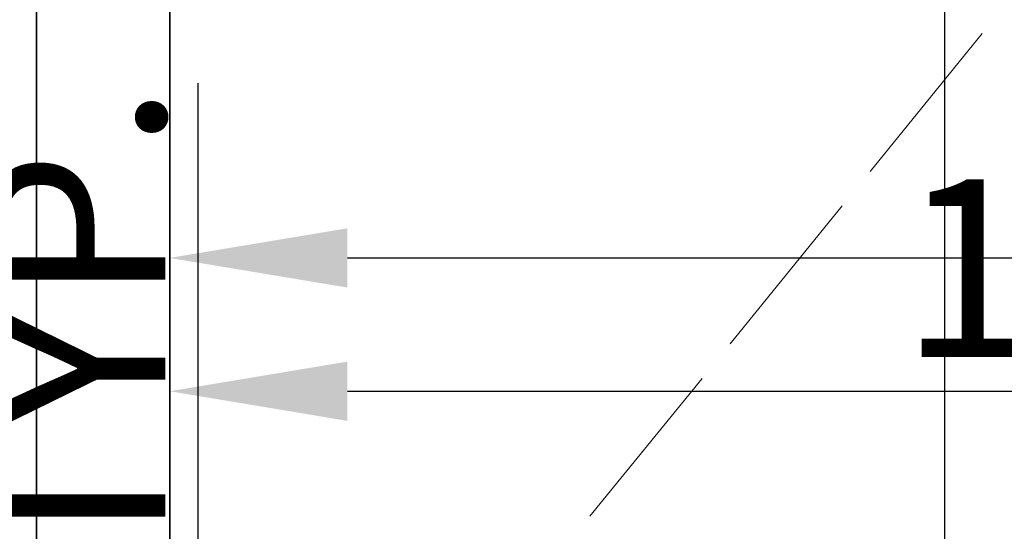
# Model space of a CAD drawing. Units: inches. Extents: x 2083 to 3317, y 1141 to 2115.
# Tile 80 of 256: x 2226 to 2292, y 1512 to 1546. Entities that reach past the tile are written whole.
import ezdxf

# ---------------------------------------------------------------- set-up
doc = ezdxf.new("R2010")
doc.units = ezdxf.units.IN
doc.linetypes.add('ACAD_ISO02W100', pattern=[15, 12, -3])
for name, color, linetype, lineweight in [('A-ANNO-DIMS', 2, 'Continuous', 18), ('A-FLOR-OPEN', 8, 'ACAD_ISO02W100', 13), ('A-WALL', 7, 'Continuous', 35)]:
    doc.layers.add(name, color=color, linetype=linetype, lineweight=lineweight)
doc.layers.add('A-WALL-PATT', color=251, linetype='Continuous', lineweight=13, true_color=0x636466)
doc.styles.get("Standard").update_dxf_attribs({"font": 'arial.ttf'})
doc.dimstyles.new('ISO-25', dxfattribs={"dimtxt": 12, "dimasz": 12, "dimexe": 1.25, "dimexo": 0.625, "dimtad": 1, "dimlunit": 3, "dimtxsty": 'Standard', "dimcen": 2.5, "dimadec": 0, "dimazin": 0, "dimtfac": 1, "dimtmove": 0, "dimatfit": 3, "dimfxl": 1, "dimarcsym": 0})

# ---------------------------------------------------------------- blocks, each defined once
blk = doc.blocks.new('*D31')
at = {"layer": 'A-ANNO-DIMS', "color": 0, "lineweight": -2, "transparency": 16777216}
for p, q in [((2237.871, 1456.649), (2237.871, 1541.915)), ((2239.393, 1444.649), (2236.621, 1444.649)), ((2237.871, 1431.548), (2237.871, 1444.649)), ((2239.393, 1431.548), (2236.621, 1431.548)), ((2237.871, 1419.548), (2237.871, 1407.548))]:
    blk.add_line(p, q, dxfattribs=at)
at = {"layer": 'A-ANNO-DIMS', "color": 0, "transparency": 16777216}
for points in [[(2235.871, 1456.649), (2239.871, 1456.649), (2237.871, 1444.649)], [(2235.871, 1419.548), (2239.871, 1419.548), (2237.871, 1431.548)]]:
    blk.add_solid(points, dxfattribs=at)
at = {"layer": 'Defpoints', "color": 0, "transparency": 16777216}
for p in [(2237.871, 1444.649), (2240.018, 1444.649), (2240.018, 1431.548)]:
    blk.add_point(p, dxfattribs=at)
at = {"layer": 'A-ANNO-DIMS', "color": 0, "transparency": 16777216, "insert": (2231.217, 1505.282), "char_height": 12, "attachment_point": 5, "rotation": 90}
blk.add_mtext('1\'-1" TYP.', dxfattribs=at)
blk = doc.blocks.new('*D45')
at = {"layer": 'A-ANNO-DIMS', "color": 0, "lineweight": -2, "transparency": 16777216}
for p, q in [((2235.96, 1478.386), (2235.96, 1531.361)), ((2418.96, 1478.386), (2418.96, 1531.361)), ((2247.96, 1530.111), (2406.96, 1530.111))]:
    blk.add_line(p, q, dxfattribs=at)
at = {"layer": 'A-ANNO-DIMS', "color": 0, "transparency": 16777216}
for points in [[(2247.96, 1532.111), (2247.96, 1528.111), (2235.96, 1530.111)], [(2406.96, 1532.111), (2406.96, 1528.111), (2418.96, 1530.111)]]:
    blk.add_solid(points, dxfattribs=at)
at = {"layer": 'Defpoints', "color": 0, "transparency": 16777216}
for p in [(2418.96, 1530.111), (2235.96, 1477.761), (2418.96, 1477.761)]:
    blk.add_point(p, dxfattribs=at)
at = {"layer": 'A-ANNO-DIMS', "color": 0, "transparency": 16777216, "insert": (2327.46, 1536.867), "char_height": 12, "attachment_point": 5}
blk.add_mtext('15\'-3"', dxfattribs=at)
blk = doc.blocks.new('*D62')
at = {"layer": 'A-ANNO-DIMS', "color": 0, "lineweight": -2, "transparency": 16777216}
for p, q in [((2235.96, 1469.386), (2235.96, 1522.361)), ((2379.96, 1469.386), (2379.96, 1522.361)), ((2247.96, 1521.111), (2367.96, 1521.111))]:
    blk.add_line(p, q, dxfattribs=at)
at = {"layer": 'A-ANNO-DIMS', "color": 0, "transparency": 16777216}
for points in [[(2247.96, 1523.111), (2247.96, 1519.111), (2235.96, 1521.111)], [(2367.96, 1523.111), (2367.96, 1519.111), (2379.96, 1521.111)]]:
    blk.add_solid(points, dxfattribs=at)
at = {"layer": 'Defpoints', "color": 0, "transparency": 16777216}
for p in [(2379.96, 1521.111), (2235.96, 1468.761), (2379.96, 1468.761)]:
    blk.add_point(p, dxfattribs=at)
at = {"layer": 'A-ANNO-DIMS', "color": 0, "transparency": 16777216, "insert": (2307.96, 1527.863), "char_height": 12, "attachment_point": 5}
blk.add_mtext('12\'-0"', dxfattribs=at)
blk = doc.blocks.new('*D64')
at = {"layer": 'A-ANNO-DIMS', "color": 0, "lineweight": -2, "transparency": 16777216}
for p, q in [((2236.585, 1702.761), (2289.56, 1702.761)), ((2288.31, 1690.761), (2288.31, 1489.761)), ((2236.585, 1477.761), (2289.56, 1477.761))]:
    blk.add_line(p, q, dxfattribs=at)
at = {"layer": 'A-ANNO-DIMS', "color": 0, "transparency": 16777216}
for points in [[(2286.31, 1690.761), (2290.31, 1690.761), (2288.31, 1702.761)], [(2286.31, 1489.761), (2290.31, 1489.761), (2288.31, 1477.761)]]:
    blk.add_solid(points, dxfattribs=at)
at = {"layer": 'Defpoints', "color": 0, "transparency": 16777216}
for p in [(2235.96, 1702.761), (2235.96, 1477.761), (2288.31, 1477.761)]:
    blk.add_point(p, dxfattribs=at)
at = {"layer": 'A-ANNO-DIMS', "color": 0, "transparency": 16777216, "insert": (2281.558, 1590.261), "char_height": 12, "attachment_point": 5, "rotation": 90}
blk.add_mtext('18\'-9"', dxfattribs=at)

msp = doc.modelspace()

# ---------------------------------------------------------------- hatches: boundary and pattern name
at = {"layer": 'A-WALL-PATT'}
h = msp.add_hatch(color=256, dxfattribs=at)
h.dxf.hatch_style = 1
h.paths.add_polyline_path([(3126.96, 2020.761), (2748.96, 2020.761), (2604.96, 2020.761), (2226.96, 2020.761), (2226.96, 1702.761), (2466.96, 1702.761), (2466.96, 1582.761), (2418.96, 1582.761), (2418.96, 1477.761), (2226.96, 1477.761), (2226.96, 1263.261), (2544.96, 1263.261), (2544.96, 1411.761), (2604.96, 1411.761), (2685.96, 1411.761), (2685.96, 1420.761), (2604.96, 1420.761), (2604.96, 1573.761), (2604.96, 1702.761), (2604.96, 2011.761), (2748.96, 2011.761), (2748.96, 1702.761), (2862.96, 1702.761), (2862.96, 1621.761), (2871.96, 1621.761), (2871.96, 1702.761), (2883.96, 1702.761), (2883.96, 1706.939, -0.026459), (2883.96, 1711.761), (2757.96, 1711.761), (2757.96, 1807.761), (2787.96, 1807.761), (2787.96, 1812.261), (2757.96, 1812.261), (2757.96, 2011.761), (2877.96, 2011.761), (2877.96, 1812.261), (2847.96, 1812.261), (2847.96, 1807.761), (2889.836, 1807.761), (2889.836, 1812.261), (2882.46, 1812.261), (2882.46, 2011.761), (3117.96, 2011.761), (3117.96, 1812.261), (2937.836, 1812.261), (2937.836, 1807.761), (2995.71, 1807.761), (2995.71, 1796.118), (3000.21, 1796.118), (3000.21, 1807.761), (3117.96, 1807.761), (3117.96, 1711.761), (3000.21, 1711.761), (3000.21, 1760.118), (2998.573, 1760.118, -0.020711), (2995.71, 1760.118), (2995.71, 1711.761), (2931.96, 1711.761), (2931.96, 1702.761), (3126.96, 1702.761)])
h.paths.add_polyline_path([(2471.46, 2011.761), (2471.46, 1810.011), (2462.717, 1810.011), (2462.717, 1805.511), (2505.96, 1805.511), (2505.96, 1810.011), (2475.96, 1810.011), (2475.96, 2011.761), (2595.96, 2011.761), (2595.96, 1810.011), (2565.96, 1810.011), (2565.96, 1805.511), (2595.96, 1805.511), (2595.96, 1711.761), (2235.96, 1711.761), (2235.96, 1805.511), (2353.71, 1805.511), (2353.71, 1796.054), (2358.21, 1796.054), (2358.21, 1805.511), (2414.717, 1805.511), (2414.717, 1810.011), (2235.96, 1810.011), (2235.96, 2011.761)], flags=16)
h.paths.add_polyline_path([(2270.205, 1994.61), (2270.205, 1970.61), (2246.205, 1970.61), (2246.205, 1994.61)], flags=0)
edge = h.paths.add_edge_path(flags=0)
edge.add_ellipse((2332.027, 1899.798), major_axis=(-3.043, 3.043), ratio=0.168252, start_angle=-161.33217, end_angle=-156.30711, ccw=False)
edge.add_ellipse((2333.082, 1898.744), major_axis=(-1.055, 1.055), ratio=0.453532, start_angle=-123.37102, end_angle=-94.15911)
edge = h.paths.add_edge_path(flags=0)
edge.add_ellipse((2332.027, 1968.876), major_axis=(3.043, 3.043), ratio=0.168252, start_angle=18.66783, end_angle=23.69289)
edge.add_spline(control_points=[(2332.926, 1970.691), (2332.227, 1970.336), (2330.894, 1969.659), (2328.413, 1970.932), (2327.204, 1967.749), (2324.71, 1969.956), (2322.533, 1967.012), (2320.013, 1971.296), (2317.68, 1968.158), (2316.041, 1967.102), (2315.427, 1966.81)], knot_values=[0, 0, 0, 0, 2.267059, 4.324559, 6.685584, 8.878641, 11.121502, 14.300359, 17.755284, 19.732645, 19.732645, 19.732645, 19.732645], degree=3, periodic=0)
edge.add_ellipse((2332.027, 1968.876), major_axis=(3.043, 3.043), ratio=0.168252, start_angle=18.66783, end_angle=23.69289, ccw=False)
edge.add_ellipse((2333.082, 1969.931), major_axis=(1.055, 1.055), ratio=0.453532, start_angle=56.62898, end_angle=85.84089, ccw=False)
edge = h.paths.add_edge_path(flags=0)
edge.add_spline(control_points=[(2296.428, 1967.988), (2293.628, 1965.336), (2287.704, 1959.727), (2299.744, 1949.996), (2294.533, 1935.669), (2290.573, 1920.604), (2293.394, 1909.974), (2296.185, 1904.967)], knot_values=[0.099185, 0.099185, 0.099185, 0.099185, 0.345301, 0.619822, 0.982653, 1.386093, 1.810555, 1.810555, 1.810555, 1.810555], degree=3, periodic=0)
edge.add_spline(control_points=[(2296.185, 1904.967), (2297.384, 1902.619), (2298.001, 1901.949), (2298.553, 1901.468)], knot_values=[0.006246, 0.006246, 0.006246, 0.006246, 0.055476, 0.055476, 0.055476, 0.055476], degree=3, periodic=0)
edge.add_spline(control_points=[(2298.553, 1901.468), (2297.259, 1900.923), (2295.225, 1900.232), (2293.06, 1900.614), (2292.101, 1900.788), (2292.09, 1900.791)], knot_values=[0.312835, 0.312835, 0.312835, 0.312835, 0.40178, 0.474987, 0.475903, 0.475903, 0.475903, 0.475903], degree=3, periodic=0)
edge.add_arc((2292.794, 1904.664), 3.937, 215.4209, 259.69818, ccw=False)
edge.add_spline(control_points=[(2289.585, 1902.382), (2289.477, 1902.535), (2289.368, 1902.688), (2289.261, 1902.841)], knot_values=[0.102872, 0.102872, 0.102872, 0.102872, 0.116896, 0.116896, 0.116896, 0.116896], degree=3, periodic=0)
edge.add_spline(control_points=[(2289.261, 1902.841), (2288.687, 1902.55), (2287.64, 1902.02), (2285.881, 1901.874), (2283.853, 1901.504), (2281.72, 1899.711), (2278.467, 1899.493), (2276.157, 1901.883), (2272.259, 1899.804), (2267.778, 1901.843), (2262.244, 1900.184), (2257.415, 1901.782), (2254.318, 1900.726), (2253.178, 1900.337)], knot_values=[0, 0, 0, 0, 1.907977, 3.477176, 5.261074, 7.972851, 11.680248, 13.717921, 16.939592, 22.789562, 27.502503, 33.595215, 37.145618, 37.145618, 37.145618, 37.145618], degree=3, periodic=0)
edge.add_line((2253.178, 1900.337), (2250.244, 1902.841))
edge.add_line((2250.244, 1902.841), (2250.244, 1965.833))
edge.add_line((2250.244, 1965.833), (2253.178, 1968.337))
edge.add_spline(control_points=[(2253.178, 1968.337), (2254.318, 1967.948), (2257.415, 1966.892), (2262.244, 1968.49), (2267.778, 1966.831), (2271.527, 1968.537), (2273.876, 1967.828), (2274.207, 1967.728)], knot_values=[0, 0, 0, 0, 0.09018, 0.244935, 0.364644, 0.513233, 0.537855, 0.537855, 0.537855, 0.537855], degree=3, periodic=0)
edge.add_arc((2274.353, 1963.793), 3.937, 72.05113, 92.12795, ccw=False)
edge.add_arc((2281.297, 1985.23), 18.596, 252.05113, 288.56572)
edge.add_arc((2292.317, 1956.029), 12.646, 71.02679, 113.77822, ccw=False)
edge = h.paths.add_edge_path(flags=0)
edge.add_spline(control_points=[(2274.899, 1951.856), (2275.066, 1951.617), (2275.233, 1951.377), (2275.398, 1951.136)], knot_values=[1.409916, 1.409916, 1.409916, 1.409916, 1.43159, 1.43159, 1.43159, 1.43159], degree=3, periodic=0)
edge.add_spline(control_points=[(2275.398, 1951.136), (2275.792, 1950.562), (2276.179, 1949.984), (2276.546, 1949.397)], knot_values=[1.358238, 1.358238, 1.358238, 1.358238, 1.409916, 1.409916, 1.409916, 1.409916], degree=3, periodic=0)
edge.add_line((2276.546, 1949.397), (2277.437, 1947.862))
edge.add_spline(control_points=[(2277.437, 1947.862), (2276.304, 1945.673), (2274.64, 1942.427), (2274.632, 1938.094), (2272.799, 1930.852), (2274.356, 1943.897), (2275.948, 1947.923), (2276.546, 1949.397)], knot_values=[0.005632, 0.005632, 0.005632, 0.005632, 0.186014, 0.266002, 0.357087, 0.59639, 0.739732, 0.739732, 0.739732, 0.739732], degree=3, periodic=0)
edge.add_spline(control_points=[(2276.546, 1949.397), (2276.179, 1949.984), (2275.792, 1950.562), (2275.398, 1951.136)], knot_values=[1.358238, 1.358238, 1.358238, 1.358238, 1.409916, 1.409916, 1.409916, 1.409916], degree=3, periodic=0)
edge.add_spline(control_points=[(2275.398, 1951.136), (2274.943, 1950.08), (2274.208, 1948.025), (2273.935, 1944.851), (2272.469, 1937.627), (2273.466, 1945.696), (2274.701, 1951.059), (2274.899, 1951.856)], knot_values=[0.104364, 0.104364, 0.104364, 0.104364, 0.189636, 0.269624, 0.36071, 0.600013, 0.644622, 0.644622, 0.644622, 0.644622], degree=3, periodic=0)
h.paths.add_polyline_path([(2269.168, 1963.128, -0.357527), (2268.171, 1960.976, -0.092561), (2268.171, 1939.436, -0.357527), (2269.168, 1937.285, -0.357527), (2267.016, 1938.282, -0.164785), (2254.686, 1938.282, -0.357527), (2252.534, 1937.285, -0.357527), (2253.531, 1939.436, -0.092561), (2253.531, 1960.976, -0.357527), (2252.534, 1963.128, -0.357527), (2254.686, 1962.131, -0.164785), (2267.016, 1962.131, -0.357527)], flags=0)
h.paths.add_polyline_path([(2248.874, 1967.802), (2248.874, 1957.028), (2249.458, 1957.028), (2249.458, 1911.647), (2248.874, 1911.647), (2248.874, 1900.873), (2246.512, 1900.873, 0.197327), (2244.15, 1902.457), (2244.15, 1966.218, 0.197327), (2246.512, 1967.802)], flags=0)
h.paths.add_polyline_path([(2269.168, 1931.389, -0.357527), (2268.171, 1929.238, -0.092561), (2268.171, 1907.698, -0.357527), (2269.168, 1905.547, -0.357527), (2267.016, 1906.544, -0.164785), (2254.686, 1906.544, -0.357527), (2252.534, 1905.547, -0.357527), (2253.531, 1907.698, -0.092561), (2253.531, 1929.238, -0.357527), (2252.534, 1931.389, -0.357527), (2254.686, 1930.392, -0.164785), (2267.016, 1930.392, -0.357527)], flags=0)
edge = h.paths.add_edge_path(flags=0)
edge.add_spline(control_points=[(2276.197, 1906.724), (2276.168, 1909.029), (2276.114, 1913.372), (2270.598, 1924.925), (2273.905, 1919.013), (2275.922, 1916.262), (2275.475, 1912.402), (2277.258, 1910.381), (2276.696, 1908.225), (2276.646, 1906.813), (2276.618, 1906.008)], knot_values=[0, 0, 0, 0, 8.61026, 16.221274, 18.843057, 23.804898, 27.440828, 29.356102, 31.203478, 33.650687, 33.650687, 33.650687, 33.650687], degree=3, periodic=0)
edge.add_spline(control_points=[(2276.618, 1906.008), (2276.623, 1905.624), (2276.498, 1904.629), (2275.442, 1903.855), (2274.937, 1903.08), (2274.859, 1902.841)], knot_values=[0.156488, 0.156488, 0.156488, 0.156488, 0.184398, 0.231376, 0.250598, 0.250598, 0.250598, 0.250598], degree=3, periodic=0)
edge.add_line((2274.859, 1902.841), (2276.506, 1902.841))
edge.add_spline(control_points=[(2276.506, 1902.841), (2276.788, 1903.085), (2277.665, 1904.125), (2278.25, 1904.341), (2277.654, 1908.527), (2278.156, 1906.228), (2278.1, 1905.286), (2278.847, 1904.069), (2277.857, 1903.415), (2277.874, 1902.991), (2277.904, 1902.841)], knot_values=[0.059574, 0.059574, 0.059574, 0.059574, 0.080753, 0.103741, 0.16972, 0.176036, 0.207137, 0.240474, 0.262341, 0.27366, 0.27366, 0.27366, 0.27366], degree=3, periodic=0)
edge.add_line((2277.904, 1902.841), (2280.03, 1902.841))
edge.add_spline(control_points=[(2280.03, 1902.841), (2279.888, 1903.088), (2279.499, 1903.982), (2280.152, 1905.939), (2278.104, 1909.658), (2279.762, 1907.185), (2280.328, 1904.875), (2280.485, 1903.49), (2281.463, 1903.249), (2281.758, 1902.936), (2281.834, 1902.841)], knot_values=[0.013856, 0.013856, 0.013856, 0.013856, 0.034874, 0.088867, 0.107879, 0.126738, 0.158714, 0.193757, 0.217487, 0.226722, 0.226722, 0.226722, 0.226722], degree=3, periodic=0)
edge.add_spline(control_points=[(2281.834, 1902.841), (2281.788, 1902.827), (2281.647, 1902.783), (2281.396, 1902.859), (2281.088, 1902.985), (2280.721, 1903.061), (2280.333, 1903.026), (2280.125, 1902.899), (2280.03, 1902.841)], knot_values=[0, 0, 0, 0, 0.14413, 0.435517, 0.749276, 1.153046, 1.548371, 1.878348, 1.878348, 1.878348, 1.878348], degree=3, periodic=0)
edge.add_line((2280.03, 1902.841), (2277.904, 1902.841))
edge.add_spline(control_points=[(2277.904, 1902.841), (2277.893, 1902.796), (2277.865, 1902.68), (2277.607, 1902.687), (2277.274, 1902.801), (2276.838, 1902.62), (2276.584, 1902.789), (2276.506, 1902.841)], knot_values=[0, 0, 0, 0, 0.127189, 0.326199, 0.628009, 1.24357, 1.515331, 1.515331, 1.515331, 1.515331], degree=3, periodic=0)
edge.add_line((2276.506, 1902.841), (2274.859, 1902.841))
edge.add_spline(control_points=[(2274.859, 1902.841), (2274.814, 1902.899), (2274.725, 1903.013), (2274.493, 1903.119), (2274.244, 1902.961), (2273.937, 1903.185), (2273.614, 1902.983), (2273.408, 1902.883), (2273.322, 1902.841)], knot_values=[0, 0, 0, 0, 0.21843, 0.436957, 0.687977, 0.990379, 1.398396, 1.69185, 1.69185, 1.69185, 1.69185], degree=3, periodic=0)
edge.add_spline(control_points=[(2273.322, 1902.841), (2273.617, 1903.446), (2274.274, 1904.538), (2276.027, 1904.574), (2276.207, 1906.584), (2276.197, 1906.724)], knot_values=[0.012227, 0.012227, 0.012227, 0.012227, 0.059472, 0.106218, 0.134458, 0.134458, 0.134458, 0.134458], degree=3, periodic=0)
h.paths.add_polyline_path([(2270.776, 1897.79), (2270.776, 1873.79), (2246.776, 1873.79), (2246.776, 1897.79)], flags=0)
h.paths.add_polyline_path([(2353.71, 1760.005), (2353.71, 1760.054), (2358.21, 1760.054, -0.033729)], flags=0)
h.paths.add_polyline_path([(2321.819, 1737.529), (2341.995, 1737.529, -0.414214), (2343.203, 1736.321), (2343.203, 1721.021, -0.414214), (2341.995, 1719.813), (2321.819, 1719.813, -0.414214), (2320.611, 1721.021), (2320.611, 1736.321, -0.414214)], flags=0)
h.paths.add_polyline_path([(2324.235, 1736.321), (2339.579, 1736.321, -0.414214), (2341.995, 1733.905), (2341.995, 1725.45, -0.414214), (2339.579, 1723.034), (2333.681, 1723.034), (2333.845, 1722.045, -0.870646), (2335.425, 1721.826, -0.767327), (2333.923, 1721.423), (2331.291, 1721.423, -0.767327), (2329.788, 1721.826, -0.870646), (2331.368, 1722.045), (2331.533, 1723.034), (2324.235, 1723.034, -0.414214), (2321.819, 1725.45), (2321.819, 1733.905, -0.414214)], flags=0)
h.paths.add_polyline_path([(2570.484, 1928.615), (2589.684, 1928.615), (2590.169, 1928.615), (2590.169, 1904.993), (2570.484, 1904.993)], flags=0)
h.paths.add_polyline_path([(2574.447, 1927.264, -1), (2572.829, 1927.264, -1)], flags=0)
h.paths.add_polyline_path([(2573.09, 1926.941), (2573.925, 1927.776), (2574.148, 1927.553), (2573.313, 1926.718)], flags=0)
h.paths.add_polyline_path([(2578.779, 1919.73, -1), (2571.592, 1919.73, -1)], flags=0)
h.paths.add_polyline_path([(2578.385, 1919.73, -1), (2571.985, 1919.73, -1)], flags=0)
h.paths.add_polyline_path([(2331.596, 1729.476, -1), (2333.618, 1729.476, -1)], flags=0)
h.paths.add_polyline_path([(2578.034, 1927.264, -1), (2576.416, 1927.264, -1)], flags=0)
h.paths.add_polyline_path([(2576.689, 1927.531), (2576.912, 1927.754), (2577.747, 1926.919), (2577.524, 1926.696)], flags=0)
h.paths.add_polyline_path([(2578.139, 1909.86, -1), (2572.232, 1909.86, -1)], flags=0)
h.paths.add_polyline_path([(2577.745, 1909.86, -1), (2572.625, 1909.86, -1)], flags=0)
h.paths.add_polyline_path([(2583.798, 1927.264, -1), (2582.179, 1927.264, -1)], flags=0)
h.paths.add_polyline_path([(2582.719, 1927.754), (2583.554, 1926.919), (2583.331, 1926.696), (2582.496, 1927.531)], flags=0)
h.paths.add_polyline_path([(2582.496, 1927.531), (2582.719, 1927.754), (2583.554, 1926.919), (2583.331, 1926.696)], flags=0)
h.paths.add_polyline_path([(2587.739, 1920.53, -1), (2581.832, 1920.53, -1)], flags=0)
h.paths.add_polyline_path([(2587.345, 1920.53, -1), (2582.225, 1920.53, -1)], flags=0)
h.paths.add_polyline_path([(2587.385, 1927.264, -1), (2585.766, 1927.264, -1)], flags=0)
h.paths.add_polyline_path([(2586.082, 1926.98), (2586.917, 1927.815), (2587.14, 1927.593), (2586.305, 1926.758)], flags=0)
h.paths.add_polyline_path([(2588.379, 1910.66, -1), (2581.192, 1910.66, -1)], flags=0)
h.paths.add_polyline_path([(2587.985, 1910.66, -1), (2581.585, 1910.66, -1)], flags=0)
h.paths.add_polyline_path([(2417.168, 1729.478), (2437.344, 1729.478, -0.414214), (2438.552, 1728.27), (2438.552, 1712.969, -0.414214), (2437.344, 1711.761), (2417.168, 1711.761, -0.414214), (2415.96, 1712.969), (2415.96, 1728.27, -0.414214)], flags=0)
h.paths.add_polyline_path([(2419.584, 1728.27), (2434.928, 1728.27, -0.414214), (2437.344, 1725.854), (2437.344, 1717.398, -0.414214), (2434.928, 1714.983), (2429.029, 1714.983), (2429.194, 1713.994, -0.870646), (2430.774, 1713.775, -0.767327), (2429.271, 1713.372), (2426.64, 1713.372, -0.767327), (2425.137, 1713.775, -0.870646), (2426.717, 1713.994), (2426.882, 1714.983), (2419.584, 1714.983, -0.414214), (2417.168, 1717.398), (2417.168, 1725.854, -0.414214)], flags=0)
h.paths.add_polyline_path([(2419.584, 1728.27), (2434.928, 1728.27, -0.414214), (2437.344, 1725.854), (2437.344, 1717.398, -0.414214), (2434.928, 1714.983), (2429.029, 1714.983), (2428.358, 1719.009), (2427.553, 1719.009), (2426.882, 1714.983), (2419.584, 1714.983, -0.414214), (2417.168, 1717.398), (2417.168, 1725.854, -0.414214)], flags=0)
h.paths.add_polyline_path([(2426.944, 1721.425, -1), (2428.967, 1721.425, -1)], flags=0)
h.paths.add_polyline_path([(2475.96, 1702.761), (2595.96, 1702.761), (2595.96, 1582.761), (2475.96, 1582.761)], flags=16)
h.paths.add_polyline_path([(2427.96, 1573.761), (2595.96, 1573.761), (2595.96, 1468.761), (2595.96, 1420.761), (2384.46, 1420.761), (2384.46, 1468.761), (2427.96, 1468.761)], flags=16)
h.paths.add_polyline_path([(2379.96, 1468.761), (2379.96, 1420.761), (2235.96, 1420.761), (2235.96, 1468.761)], flags=16)
h.paths.add_polyline_path([(2317.816, 1466.696), (2337.992, 1466.696, -0.414214), (2339.2, 1465.488), (2339.2, 1450.187, -0.414214), (2337.992, 1448.979), (2317.816, 1448.979, -0.414214), (2316.608, 1450.187), (2316.608, 1465.488, -0.414214)], flags=0)
h.paths.add_polyline_path([(2320.232, 1465.488), (2335.576, 1465.488, -0.414214), (2337.992, 1463.072), (2337.992, 1454.616, -0.414214), (2335.576, 1452.2), (2329.677, 1452.2), (2329.842, 1451.212, -0.870646), (2331.422, 1450.992, -0.767327), (2329.92, 1450.59), (2327.288, 1450.59, -0.767327), (2325.785, 1450.992, -0.870646), (2327.365, 1451.212), (2327.53, 1452.2), (2320.232, 1452.2, -0.414214), (2317.816, 1454.616), (2317.816, 1463.072, -0.414214)], flags=0)
h.paths.add_polyline_path([(2320.232, 1465.488), (2335.576, 1465.488, -0.414214), (2337.992, 1463.072), (2337.992, 1454.616, -0.414214), (2335.576, 1452.2), (2329.677, 1452.2), (2329.006, 1456.227), (2328.201, 1456.227), (2327.53, 1452.2), (2320.232, 1452.2, -0.414214), (2317.816, 1454.616), (2317.816, 1463.072, -0.414214)], flags=0)
h.paths.add_polyline_path([(2327.593, 1458.643, -1), (2329.615, 1458.643, -1)], flags=0)
h.paths.add_polyline_path([(2244.412, 1433.34), (2241.921, 1433.34, -0.414214), (2240.018, 1435.244), (2240.018, 1440.953, -0.414211), (2241.921, 1442.856), (2244.412, 1442.856, -1.976472)], flags=0)
h.paths.add_polyline_path([(2245.357, 1434.398, -0.414214), (2245.357, 1441.799, -2.144098)], flags=0)
h.paths.add_polyline_path([(2535.96, 1416.261), (2535.96, 1272.261), (2235.96, 1272.261), (2235.96, 1416.261)], flags=16)
h.paths.add_polyline_path([(2260.12, 1384.293), (2260.12, 1362.039), (2237.865, 1362.039), (2237.865, 1384.293)], flags=0)
edge = h.paths.add_edge_path(flags=0)
edge.add_line((2318.252, 1362.093), (2318.146, 1362.001))
edge.add_ellipse((2317.445, 1360.431), major_axis=(2.822, 2.822), ratio=0.168252, start_angle=18.66783, end_angle=20.94813, ccw=False)
edge.add_ellipse((2318.423, 1361.409), major_axis=(0.978, 0.978), ratio=0.453532, start_angle=56.62898, end_angle=70.2262, ccw=False)
edge = h.paths.add_edge_path(flags=0)
edge.add_line((2319.107, 1295.571), (2319.015, 1295.677))
edge.add_ellipse((2317.445, 1296.378), major_axis=(-2.822, 2.822), ratio=0.168252, start_angle=-161.33217, end_angle=-159.05187, ccw=False)
edge.add_ellipse((2318.423, 1295.4), major_axis=(-0.978, 0.978), ratio=0.453532, start_angle=-123.37102, end_angle=-109.7738)
edge = h.paths.add_edge_path(flags=0)
edge.add_spline(control_points=[(2284.21, 1301.17), (2284.581, 1300.445), (2284.891, 1299.892), (2285.16, 1299.461)], knot_values=[0.039066, 0.039066, 0.039066, 0.039066, 0.055476, 0.055476, 0.055476, 0.055476], degree=3, periodic=0)
edge.add_line((2285.16, 1299.461), (2284.21, 1301.17))
edge = h.paths.add_edge_path(flags=0)
edge.add_line((2280.412, 1297.298), (2283.37, 1297.036))
edge.add_line((2283.37, 1297.036), (2286.406, 1297.926))
edge.add_spline(control_points=[(2286.406, 1297.926), (2285.305, 1297.463), (2284.345, 1297.129), (2283.37, 1297.036)], knot_values=[0.394369, 0.394369, 0.394369, 0.394369, 0.475903, 0.475903, 0.475903, 0.475903], degree=3, periodic=0)
edge.add_spline(control_points=[(2283.37, 1297.036), (2283.281, 1297.028), (2282.316, 1296.957), (2281.313, 1297.134), (2280.423, 1297.296), (2280.412, 1297.298)], knot_values=[0.312835, 0.312835, 0.312835, 0.312835, 0.320246, 0.393453, 0.394369, 0.394369, 0.394369, 0.394369], degree=3, periodic=0)
edge = h.paths.add_edge_path(flags=0)
edge.add_line((2284.436, 1359.607), (2280.446, 1355.328))
edge.add_line((2280.446, 1355.328), (2279.58, 1351.018))
edge.add_line((2279.58, 1351.018), (2282.413, 1346.58))
edge.add_spline(control_points=[(2282.413, 1346.58), (2283.153, 1345.589), (2284.253, 1344.029), (2284.801, 1342.387), (2284.935, 1341.806)], knot_values=[1.240098, 1.240098, 1.240098, 1.240098, 1.332892, 1.382712, 1.382712, 1.382712, 1.382712], degree=3, periodic=0)
edge.add_spline(control_points=[(2284.935, 1341.806), (2285.319, 1340.141), (2285.233, 1338.409), (2284.91, 1336.654)], knot_values=[1.097484, 1.097484, 1.097484, 1.097484, 1.240098, 1.240098, 1.240098, 1.240098], degree=3, periodic=0)
edge.add_spline(control_points=[(2284.91, 1336.654), (2284.587, 1334.899), (2284.027, 1333.12), (2283.463, 1331.361)], knot_values=[0.95487, 0.95487, 0.95487, 0.95487, 1.097484, 1.097484, 1.097484, 1.097484], degree=3, periodic=0)
edge.add_line((2283.463, 1331.361), (2281.89, 1326.153))
edge.add_line((2281.89, 1326.153), (2280.756, 1321.056))
edge.add_line((2280.756, 1321.056), (2280.299, 1316.002))
edge.add_line((2280.299, 1316.002), (2280.716, 1310.95))
edge.add_line((2280.716, 1310.95), (2282.028, 1305.972))
edge.add_line((2282.028, 1305.972), (2284.21, 1301.17))
edge.add_spline(control_points=[(2284.21, 1301.17), (2283.341, 1302.73), (2282.612, 1304.336), (2282.028, 1305.972)], knot_values=[0.099185, 0.099185, 0.099185, 0.099185, 0.241799, 0.241799, 0.241799, 0.241799], degree=3, periodic=0)
edge.add_spline(control_points=[(2282.028, 1305.972), (2281.444, 1307.608), (2281.005, 1309.273), (2280.716, 1310.95)], knot_values=[0.241799, 0.241799, 0.241799, 0.241799, 0.384413, 0.384413, 0.384413, 0.384413], degree=3, periodic=0)
edge.add_spline(control_points=[(2280.716, 1310.95), (2280.433, 1312.588), (2280.289, 1314.277), (2280.299, 1315.962), (2280.299, 1316.002)], knot_values=[0.384413, 0.384413, 0.384413, 0.384413, 0.523647, 0.527028, 0.527028, 0.527028, 0.527028], degree=3, periodic=0)
edge.add_spline(control_points=[(2280.299, 1316.002), (2280.312, 1317.687), (2280.478, 1319.368), (2280.756, 1321.056)], knot_values=[0.527028, 0.527028, 0.527028, 0.527028, 0.669642, 0.669642, 0.669642, 0.669642], degree=3, periodic=0)
edge.add_spline(control_points=[(2280.756, 1321.056), (2281.035, 1322.744), (2281.426, 1324.44), (2281.89, 1326.153)], knot_values=[0.669642, 0.669642, 0.669642, 0.669642, 0.812256, 0.812256, 0.812256, 0.812256], degree=3, periodic=0)
edge.add_spline(control_points=[(2281.89, 1326.153), (2282.264, 1327.533), (2282.788, 1329.262), (2283.353, 1331.018), (2283.463, 1331.361)], knot_values=[0.812256, 0.812256, 0.812256, 0.812256, 0.927087, 0.95487, 0.95487, 0.95487, 0.95487], degree=3, periodic=0)
edge.add_line((2283.463, 1331.361), (2284.91, 1336.654))
edge.add_line((2284.91, 1336.654), (2284.935, 1341.806))
edge.add_line((2284.935, 1341.806), (2282.413, 1346.58))
edge.add_spline(control_points=[(2282.413, 1346.58), (2281.275, 1348.104), (2280.078, 1349.57), (2279.58, 1351.018)], knot_values=[1.382712, 1.382712, 1.382712, 1.382712, 1.525326, 1.525326, 1.525326, 1.525326], degree=3, periodic=0)
edge.add_spline(control_points=[(2279.58, 1351.018), (2279.443, 1351.415), (2279.136, 1352.857), (2279.735, 1354.29), (2280.446, 1355.328)], knot_values=[1.525326, 1.525326, 1.525326, 1.525326, 1.564439, 1.667941, 1.667941, 1.667941, 1.667941], degree=3, periodic=0)
edge.add_spline(control_points=[(2280.446, 1355.328), (2281.426, 1356.758), (2282.931, 1358.183), (2284.436, 1359.607)], knot_values=[1.667941, 1.667941, 1.667941, 1.667941, 1.810555, 1.810555, 1.810555, 1.810555], degree=3, periodic=0)
edge.add_arc((2280.623, 1348.518), 11.726, 71.02679, 113.77822)
edge.add_arc((2270.405, 1375.595), 17.244, 252.05113, 288.56572, ccw=False)
edge.add_arc((2263.966, 1355.718), 3.651, 72.05113, 92.12795)
edge.add_arc((2263.966, 1355.718), 3.651, 92.12795, 177.98513)
edge.add_spline(control_points=[(2260.318, 1355.846), (2260.26, 1354.221), (2260.551, 1350.187), (2262.999, 1346.766), (2264.473, 1344.649)], knot_values=[1.43159, 1.43159, 1.43159, 1.43159, 1.564144, 1.770695, 1.770695, 1.770695, 1.770695], degree=3, periodic=0)
edge.add_line((2264.473, 1344.649), (2264.936, 1343.983))
edge.add_spline(control_points=[(2263.801, 1340.248), (2263.843, 1340.514), (2264.067, 1341.756), (2264.513, 1343.002), (2264.935, 1343.981)], knot_values=[0.53657, 0.53657, 0.53657, 0.53657, 0.559349, 0.644622, 0.644622, 0.644622, 0.644622], degree=3, periodic=0)
edge.add_spline(control_points=[(2264.935, 1343.981), (2265.118, 1343.715), (2265.299, 1343.448), (2265.477, 1343.179)], knot_values=[1.384077, 1.384077, 1.384077, 1.384077, 1.409916, 1.409916, 1.409916, 1.409916], degree=3, periodic=0)
edge.add_spline(control_points=[(2265.477, 1343.179), (2265.655, 1342.911), (2265.829, 1342.641), (2265.999, 1342.369)], knot_values=[1.358238, 1.358238, 1.358238, 1.358238, 1.384077, 1.384077, 1.384077, 1.384077], degree=3, periodic=0)
edge.add_line((2265.999, 1342.369), (2266.826, 1340.946))
edge.add_spline(control_points=[(2266.826, 1340.946), (2268.894, 1337.09), (2271.398, 1325.843), (2270.516, 1310.569), (2275.919, 1301.861), (2277.79, 1299.199)], knot_values=[0.116896, 0.116896, 0.116896, 0.116896, 0.472987, 1.050969, 1.313793, 1.313793, 1.313793, 1.313793], degree=3, periodic=0)
edge.add_spline(control_points=[(2277.79, 1299.199), (2277.839, 1299.128), (2277.889, 1299.057), (2277.94, 1298.987)], knot_values=[0.109884, 0.109884, 0.109884, 0.109884, 0.116896, 0.116896, 0.116896, 0.116896], degree=3, periodic=0)
edge.add_line((2277.94, 1298.987), (2277.789, 1299.199))
edge.add_spline(control_points=[(2277.789, 1299.199), (2277.257, 1298.929), (2276.286, 1298.438), (2275.039, 1298.334), (2274.383, 1298.239), (2274.215, 1298.209)], knot_values=[33.12187, 33.12187, 33.12187, 33.12187, 35.029056, 36.598255, 37.144827, 37.144827, 37.144827, 37.144827], degree=3, periodic=0)
edge.add_line((2274.215, 1298.209), (2273.073, 1297.893))
edge.add_spline(control_points=[(2273.073, 1297.893), (2272.323, 1297.58), (2271.039, 1296.511), (2269.248, 1296.226), (2268.423, 1296.375)], knot_values=[26.532584, 26.532584, 26.532584, 26.532584, 29.198919, 31.839101, 31.839101, 31.839101, 31.839101], degree=3, periodic=0)
edge.add_line((2268.423, 1296.375), (2263.879, 1297.458))
edge.add_spline(control_points=[(2263.879, 1297.458), (2263.556, 1297.359), (2261.86, 1296.839), (2260.239, 1297.282), (2258.933, 1297.516)], knot_values=[15.919551, 15.919551, 15.919551, 15.919551, 16.939592, 21.226067, 21.226067, 21.226067, 21.226067], degree=3, periodic=0)
edge.add_line((2258.933, 1297.516), (2254.055, 1297.329))
edge.add_spline(control_points=[(2254.055, 1297.329), (2253.756, 1297.296), (2252.114, 1297.165), (2250.462, 1297.544), (2249.13, 1297.668)], knot_values=[5.306517, 5.306517, 5.306517, 5.306517, 6.276435, 10.613034, 10.613034, 10.613034, 10.613034], degree=3, periodic=0)
edge.add_line((2249.13, 1297.668), (2244.332, 1296.878))
edge.add_line((2244.332, 1296.878), (2241.611, 1299.199))
edge.add_line((2241.611, 1299.199), (2241.611, 1357.609))
edge.add_line((2241.611, 1357.609), (2244.332, 1359.931))
edge.add_line((2244.332, 1359.931), (2252.729, 1359.543))
edge.add_spline(control_points=[(2252.729, 1359.543), (2252.871, 1359.546), (2253.306, 1359.548), (2253.74, 1359.514), (2254.032, 1359.482)], knot_values=[0.233291, 0.233291, 0.233291, 0.233291, 0.244935, 0.268927, 0.268927, 0.268927, 0.268927], degree=3, periodic=0)
edge.add_line((2254.032, 1359.482), (2259.587, 1359.416))
edge.add_spline(control_points=[(2259.587, 1359.416), (2260.677, 1359.629), (2262.073, 1359.897), (2263.524, 1359.459), (2263.83, 1359.366)], knot_values=[0.422516, 0.422516, 0.422516, 0.422516, 0.513233, 0.537855, 0.537855, 0.537855, 0.537855], degree=3, periodic=0)
edge.add_arc((2263.966, 1355.718), 3.651, 72.05113, 92.12795, ccw=False)
edge.add_arc((2270.405, 1375.595), 17.244, 252.05113, 288.56572)
edge.add_arc((2280.623, 1348.518), 11.726, 71.02679, 113.77822, ccw=False)
h.paths.add_polyline_path([(2240.341, 1359.435), (2240.341, 1349.444), (2240.882, 1349.444), (2240.882, 1307.365), (2240.341, 1307.365), (2240.341, 1297.374), (2238.15, 1297.374, 0.197327), (2235.96, 1298.843), (2235.96, 1357.966, 0.197327), (2238.15, 1359.435)], flags=0)
h.paths.add_polyline_path([(2259.158, 1355.101, -0.357527), (2258.233, 1353.106, -0.092561), (2258.233, 1333.133, -0.357527), (2259.158, 1331.138, -0.357527), (2257.163, 1332.062, -0.164785), (2245.729, 1332.062, -0.357527), (2243.735, 1331.138, -0.357527), (2244.659, 1333.133, -0.092561), (2244.659, 1353.106, -0.357527), (2243.735, 1355.101, -0.357527), (2245.729, 1354.176, -0.164785), (2257.163, 1354.176, -0.357527)], flags=0)
edge = h.paths.add_edge_path(flags=0)
edge.add_line((2265.999, 1342.369), (2266.826, 1340.946))
edge.add_line((2266.826, 1340.946), (2265.308, 1337.814))
edge.add_line((2265.308, 1337.814), (2264.358, 1334.653))
edge.add_line((2264.358, 1334.653), (2264.262, 1333.8))
edge.add_spline(control_points=[(2264.262, 1333.8), (2264.208, 1333.187), (2264.162, 1332.366), (2264.007, 1331.414), (2263.969, 1331.202)], knot_values=[0.464444, 0.464444, 0.464444, 0.464444, 0.516691, 0.531608, 0.531608, 0.531608, 0.531608], degree=3, periodic=0)
edge.add_spline(control_points=[(2263.969, 1331.202), (2263.775, 1330.119), (2263.424, 1328.791), (2263.257, 1328.531), (2263.234, 1328.515)], knot_values=[0.372682, 0.372682, 0.372682, 0.372682, 0.44885, 0.464444, 0.464444, 0.464444, 0.464444], degree=3, periodic=0)
edge.add_spline(control_points=[(2263.234, 1328.515), (2263.096, 1328.42), (2263.131, 1329.301), (2263.275, 1330.616)], knot_values=[0.280919, 0.280919, 0.280919, 0.280919, 0.372682, 0.372682, 0.372682, 0.372682], degree=3, periodic=0)
edge.add_spline(control_points=[(2263.275, 1330.616), (2263.419, 1331.93), (2263.672, 1333.677), (2263.97, 1335.315)], knot_values=[0.189157, 0.189157, 0.189157, 0.189157, 0.280919, 0.280919, 0.280919, 0.280919], degree=3, periodic=0)
edge.add_spline(control_points=[(2263.97, 1335.315), (2264.1, 1336.032), (2264.419, 1337.622), (2264.755, 1338.864), (2264.947, 1339.491)], knot_values=[0.097394, 0.097394, 0.097394, 0.097394, 0.137578, 0.189157, 0.189157, 0.189157, 0.189157], degree=3, periodic=0)
edge.add_spline(control_points=[(2264.947, 1339.491), (2265.29, 1340.606), (2265.644, 1341.494), (2265.999, 1342.369)], knot_values=[0.005632, 0.005632, 0.005632, 0.005632, 0.097394, 0.097394, 0.097394, 0.097394], degree=3, periodic=0)
h.paths.add_polyline_path([(2259.158, 1325.671, -0.357527), (2258.233, 1323.676, -0.092561), (2258.233, 1303.703, -0.357527), (2259.158, 1301.708, -0.357527), (2257.163, 1302.633, -0.164785), (2245.729, 1302.633, -0.357527), (2243.735, 1301.708, -0.357527), (2244.659, 1303.703, -0.092561), (2244.659, 1323.676, -0.357527), (2243.735, 1325.671, -0.357527), (2245.729, 1324.747, -0.164785), (2257.163, 1324.747, -0.357527)], flags=0)
edge = h.paths.add_edge_path(flags=0)
edge.add_spline(control_points=[(2261.709, 1317.311), (2261.679, 1317.418), (2261.762, 1317.389), (2262.491, 1316.09), (2262.962, 1315.301)], knot_values=[14.955861, 14.955861, 14.955861, 14.955861, 16.221274, 18.694826, 18.694826, 18.694826, 18.694826], degree=3, periodic=0)
edge.add_spline(control_points=[(2262.962, 1315.301), (2262.99, 1315.254), (2263.702, 1314.067), (2264.349, 1313.127), (2264.73, 1312.164)], knot_values=[18.694826, 18.694826, 18.694826, 18.694826, 18.843057, 22.433791, 22.433791, 22.433791, 22.433791], degree=3, periodic=0)
edge.add_spline(control_points=[(2264.73, 1312.164), (2264.876, 1311.796), (2265.177, 1310.77), (2265.143, 1309.559), (2265.248, 1308.824)], knot_values=[22.433791, 22.433791, 22.433791, 22.433791, 23.804898, 26.172756, 26.172756, 26.172756, 26.172756], degree=3, periodic=0)
edge.add_line((2265.248, 1308.824), (2265.851, 1307.172))
edge.add_spline(control_points=[(2265.851, 1307.172), (2266.065, 1306.822), (2266.384, 1306.332), (2266.424, 1305.781), (2266.42, 1305.611)], knot_values=[28.062562, 28.062562, 28.062562, 28.062562, 29.356102, 29.911721, 29.911721, 29.911721, 29.911721], degree=3, periodic=0)
edge.add_spline(control_points=[(2266.42, 1305.611), (2266.416, 1305.433), (2266.394, 1305.25), (2266.365, 1305.066)], knot_values=[29.911721, 29.911721, 29.911721, 29.911721, 30.497837, 30.497837, 30.497837, 30.497837], degree=3, periodic=0)
edge.add_line((2266.365, 1305.066), (2266.066, 1302.136))
edge.add_spline(control_points=[(2266.066, 1302.136), (2266.071, 1301.78), (2265.998, 1301.2), (2265.663, 1300.759), (2265.509, 1300.586)], knot_values=[0.156488, 0.156488, 0.156488, 0.156488, 0.184398, 0.203543, 0.203543, 0.203543, 0.203543], degree=3, periodic=0)
edge.add_line((2265.509, 1300.586), (2264.435, 1299.199))
edge.add_line((2264.435, 1299.199), (2265.962, 1299.199))
edge.add_line((2265.962, 1299.199), (2267.336, 1301.175))
edge.add_line((2267.336, 1301.175), (2267.312, 1301.986))
edge.add_spline(control_points=[(2267.312, 1301.986), (2267.261, 1302.862), (2267.16, 1303.737), (2267.271, 1303.326)], knot_values=[0.126229, 0.126229, 0.126229, 0.126229, 0.166617, 0.166617, 0.166617, 0.166617], degree=3, periodic=0)
edge.add_spline(control_points=[(2267.271, 1303.326), (2267.28, 1303.294), (2267.31, 1303.175), (2267.373, 1302.884), (2267.406, 1302.683), (2267.418, 1302.601)], knot_values=[0.166617, 0.166617, 0.166617, 0.166617, 0.16972, 0.176036, 0.180765, 0.180765, 0.180765, 0.180765], degree=3, periodic=0)
edge.add_spline(control_points=[(2267.744, 1300.988), (2267.688, 1301.151), (2267.481, 1301.657), (2267.484, 1302.145), (2267.418, 1302.601)], knot_values=[0.180765, 0.180765, 0.180765, 0.180765, 0.193767, 0.220139, 0.220139, 0.220139, 0.220139], degree=3, periodic=0)
edge.add_line((2267.418, 1302.601), (2267.744, 1300.988))
edge.add_spline(control_points=[(2267.744, 1300.988), (2267.832, 1300.732), (2267.932, 1300.31), (2267.555, 1299.975), (2267.429, 1299.829)], knot_values=[0.220139, 0.220139, 0.220139, 0.220139, 0.240474, 0.25489, 0.25489, 0.25489, 0.25489], degree=3, periodic=0)
edge.add_line((2267.429, 1299.829), (2267.258, 1299.199))
edge.add_line((2267.258, 1299.199), (2269.23, 1299.199))
edge.add_spline(control_points=[(2269.23, 1299.199), (2269.099, 1299.429), (2268.843, 1300.016), (2269.012, 1300.916), (2268.947, 1301.661)], knot_values=[0.013856, 0.013856, 0.013856, 0.013856, 0.034874, 0.067073, 0.067073, 0.067073, 0.067073], degree=3, periodic=0)
edge.add_line((2268.947, 1301.661), (2268.432, 1303.603))
edge.add_spline(control_points=[(2268.432, 1303.603), (2268.176, 1304.192), (2267.596, 1305.251), (2268.041, 1304.623), (2268.251, 1304.282)], knot_values=[0.090155, 0.090155, 0.090155, 0.090155, 0.107879, 0.120289, 0.120289, 0.120289, 0.120289], degree=3, periodic=0)
edge.add_spline(control_points=[(2268.251, 1304.282), (2268.361, 1304.105), (2269.058, 1302.918), (2269.383, 1301.59), (2269.521, 1300.776), (2269.575, 1300.556)], knot_values=[0.120289, 0.120289, 0.120289, 0.120289, 0.126738, 0.158714, 0.173506, 0.173506, 0.173506, 0.173506], degree=3, periodic=0)
edge.add_line((2269.575, 1300.556), (2270.686, 1299.421))
edge.add_spline(control_points=[(2270.686, 1299.421), (2270.767, 1299.357), (2270.838, 1299.281), (2270.903, 1299.199)], knot_values=[0.21816, 0.21816, 0.21816, 0.21816, 0.226722, 0.226722, 0.226722, 0.226722], degree=3, periodic=0)
edge.add_line((2270.937, 1299.193), (2270.903, 1299.199))
edge.add_spline(control_points=[(2270.903, 1299.199), (2270.86, 1299.186), (2270.73, 1299.146), (2270.496, 1299.216), (2270.272, 1299.308), (2270.121, 1299.348), (2270.063, 1299.36)], knot_values=[0.939174, 0.939174, 0.939174, 0.939174, 1.083304, 1.374691, 1.68845, 1.878348, 1.878348, 1.878348, 1.878348], degree=3, periodic=0)
edge.add_line((2270.063, 1299.36), (2269.23, 1299.199))
edge.add_line((2269.23, 1299.199), (2267.258, 1299.199))
edge.add_spline(control_points=[(2267.258, 1299.199), (2267.248, 1299.157), (2267.223, 1299.05), (2266.984, 1299.057), (2266.809, 1299.116), (2266.677, 1299.109), (2266.637, 1299.105)], knot_values=[0.757665, 0.757665, 0.757665, 0.757665, 0.884854, 1.083864, 1.385675, 1.515331, 1.515331, 1.515331, 1.515331], degree=3, periodic=0)
edge.add_spline(control_points=[(2266.637, 1299.105), (2266.485, 1299.089), (2266.236, 1299.017), (2266.035, 1299.151), (2265.962, 1299.199)], knot_values=[0, 0, 0, 0, 0.485905, 0.757665, 0.757665, 0.757665, 0.757665], degree=3, periodic=0)
edge.add_line((2265.962, 1299.199), (2264.435, 1299.199))
edge.add_line((2264.435, 1299.199), (2263.858, 1299.367))
edge.add_spline(control_points=[(2263.858, 1299.367), (2263.819, 1299.371), (2263.78, 1299.386), (2263.74, 1299.402)], knot_values=[0.845925, 0.845925, 0.845925, 0.845925, 0.978627, 0.978627, 0.978627, 0.978627], degree=3, periodic=0)
edge.add_line((2263.722, 1299.396), (2263.01, 1299.199))
edge.add_spline(control_points=[(2263.01, 1299.199), (2263.246, 1299.683), (2263.506, 1300.128), (2263.873, 1300.408)], knot_values=[0.012227, 0.012227, 0.012227, 0.012227, 0.052971, 0.052971, 0.052971, 0.052971], degree=3, periodic=0)
edge.add_spline(control_points=[(2263.873, 1300.408), (2263.932, 1300.453), (2264.084, 1300.553), (2264.255, 1300.624), (2264.36, 1300.665)], knot_values=[0.052971, 0.052971, 0.052971, 0.052971, 0.059472, 0.069086, 0.069086, 0.069086, 0.069086], degree=3, periodic=0)
edge.add_line((2264.36, 1300.665), (2265.142, 1301.078))
edge.add_line((2265.142, 1301.078), (2265.676, 1302.8))
edge.add_line((2265.676, 1302.8), (2265.541, 1305.704))
edge.add_line((2265.541, 1305.704), (2264.803, 1309.328))
edge.add_line((2264.803, 1309.328), (2263.041, 1314.092))
edge.add_spline(control_points=[(2263.041, 1314.092), (2262.384, 1315.671), (2261.796, 1316.998), (2261.709, 1317.311)], knot_values=[11.216896, 11.216896, 11.216896, 11.216896, 14.955861, 14.955861, 14.955861, 14.955861], degree=3, periodic=0)
h.paths.add_polyline_path([(2871.96, 1416.261), (2895.91, 1416.261), (2895.91, 1420.761), (2871.96, 1420.761), (2871.96, 1501.761), (2862.96, 1501.761), (2862.96, 1420.761), (2805.96, 1420.761), (2805.96, 1411.761), (2862.96, 1411.761), (2862.96, 1263.261), (3126.96, 1263.261), (3126.96, 1411.761), (3126.96, 1486.761), (2943.96, 1486.761), (2943.96, 1477.761), (2967.86, 1477.761), (2967.86, 1420.761), (2943.91, 1420.761), (2943.91, 1416.261), (3117.96, 1416.261), (3117.96, 1420.761), (2972.36, 1420.761), (2972.36, 1477.761), (3117.96, 1477.761), (3117.96, 1420.761), (3117.96, 1272.261), (2871.96, 1272.261)], flags=0)
h.paths.add_polyline_path([(2457.126, 1485.943), (2527.603, 1485.943), (2527.603, 1537.636), (2457.126, 1537.636)], flags=8)
h.paths.add_polyline_path([(2481.005, 1609.982), (2590.766, 1609.982), (2590.766, 1682.003), (2481.005, 1682.003)], flags=8)
h.paths.add_polyline_path([(2483.085, 1729.127), (2553.562, 1729.127), (2553.562, 1780.82), (2483.085, 1780.82)], flags=8)

# ---------------------------------------------------------------- linework, layer by layer
at = {"layer": 'A-FLOR-OPEN'}
msp.add_line((2235.96, 1477.761), (2418.96, 1702.761), dxfattribs=at)
at = {"layer": 'A-WALL'}
for p, q in [((2226.96, 1702.761), (2226.96, 1263.261)), ((2235.96, 1702.761), (2235.96, 1477.761)), ((2235.96, 1702.761), (2235.96, 1477.761))]:
    msp.add_line(p, q, dxfattribs=at)

# ---------------------------------------------------------------- dimensions: what is measured, and where the dimension line sits
at = {"layer": 'A-ANNO-DIMS'}
dim = msp.add_linear_dim(base=(2288.31, 1477.761), p1=(2235.96, 1702.761), p2=(2235.96, 1477.761), angle=270, dimstyle='ISO-25', override={"dimdec": 1, "dimlfac": 1, "dimrnd": 0, "dimzin": 1, "dimdsep": 46, "dimlunit": 4, "dimfrac": 2}, dxfattribs=at)
dim.commit()
dim.dimension.update_dxf_attribs({"geometry": '*D64', "text_midpoint": (2281.558, 1590.261)})
for base, p1, p2, picture, middle in [((2418.96, 1530.111), (2235.96, 1477.761), (2418.96, 1477.761), '*D45', (2327.46, 1536.867)), ((2379.96, 1521.111), (2235.96, 1468.761), (2379.96, 1468.761), '*D62', (2307.96, 1527.863))]:
    dim = msp.add_linear_dim(base=base, p1=p1, p2=p2, dimstyle='ISO-25', override={"dimdec": 1, "dimlfac": 1, "dimrnd": 0, "dimzin": 1, "dimdsep": 46, "dimlunit": 4, "dimfrac": 2}, dxfattribs=at)
    dim.commit()
    dim.dimension.update_dxf_attribs({"geometry": picture, "text_midpoint": middle})
dim = msp.add_linear_dim(base=(2237.871, 1444.649), p1=(2240.018, 1431.548), p2=(2240.018, 1444.649), angle=90, text='<> TYP.', dimstyle='ISO-25', override={"dimdec": 1, "dimlfac": 1, "dimrnd": 0, "dimzin": 1, "dimdsep": 46, "dimlunit": 4, "dimfrac": 2}, dxfattribs=at)
dim.commit()
dim.dimension.update_dxf_attribs({"geometry": '*D31', "text_midpoint": (2231.217, 1505.282)})

doc.saveas('drawing.dxf')
